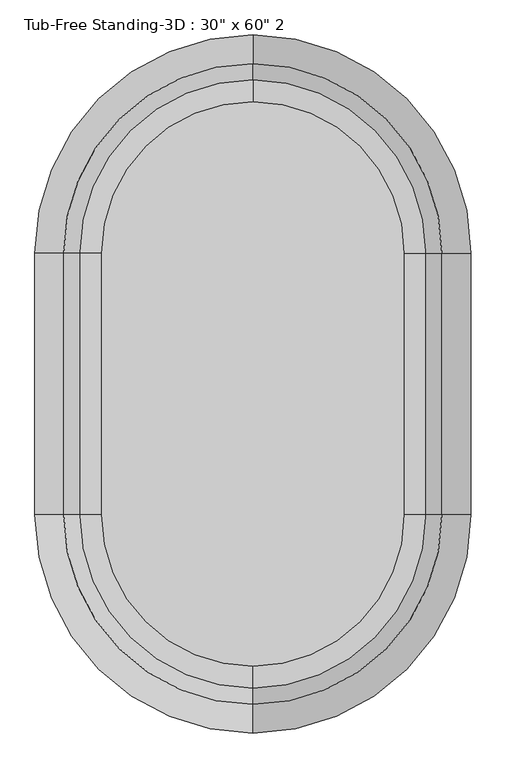
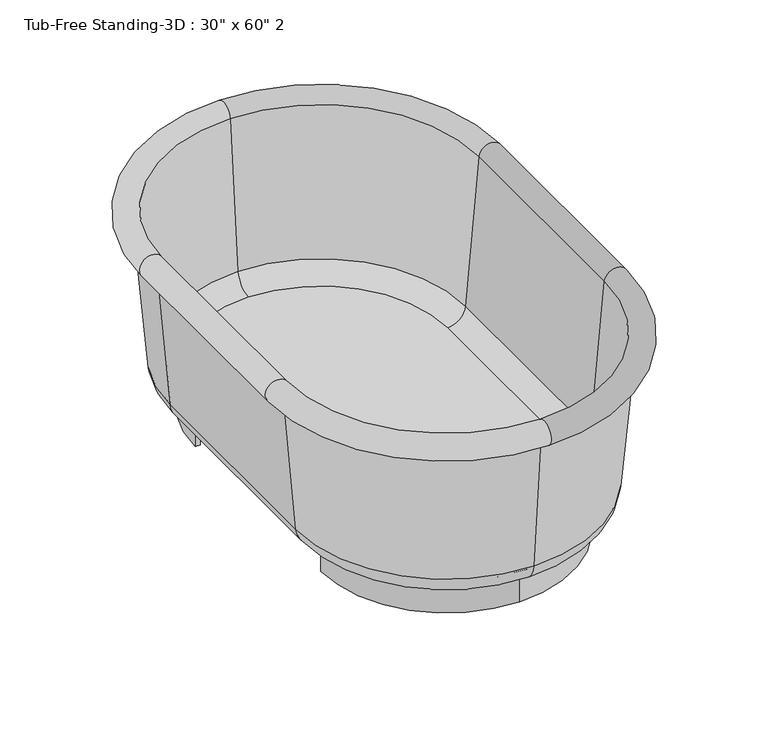
"""IFC4 building model written with IfcOpenShell, lengths in millimetres: flow terminal geometry."""

from ifc_helpers import new_model, si_unit, point, frame, frame_2d, origin, origin_with_axes, place, context, project, spatial, polyline, circle_curve, ellipse_curve, trimmed, segment, composite_curve, outline, extrude, source, transform, mapped, element, save
from ifc_brep_helpers import plane_surface, cylinder_surface, revolved_surface, advanced_brep


def flow_terminal_04541809(model_context):
    return source(origin(), model_context, "Body", "SolidModel", [
        extrude(outline(composite_curve([segment(trimmed(circle_curve(frame_2d((0.0, 228.6)), 254.0), [point((0.0, 482.6))], [point((-254.0, 228.6))], True, "CARTESIAN"), True, "CONTINUOUS"), segment(polyline([(-254.0, 228.6), (-264.2824236, 228.6)]), True, "CONTINUOUS"), segment(trimmed(circle_curve(frame_2d((0.0, 228.6)), 264.2824236), [point((-264.2824236, 228.6))], [point((0.0, 492.8824236))], False, "CARTESIAN"), True, "CONTINUOUS"), segment(trimmed(circle_curve(frame_2d((0.0, 228.6)), 264.2824236), [point((0.0, 492.8824236))], [point((264.2824236, 228.6))], False, "CARTESIAN"), True, "CONTINUOUS"), segment(polyline([(264.2824236, 228.6), (254.0, 228.6)]), True, "CONTINUOUS"), segment(trimmed(circle_curve(frame_2d((0.0, 228.6)), 254.0), [point((254.0, 228.6))], [point((0.0, 482.6))], True, "CARTESIAN"), True, "CONTINUOUS")], self_intersect=False)), origin_with_axes(), (0.0, 0.0, 1.0), 63.5),
        extrude(outline(composite_curve([segment(trimmed(circle_curve(frame_2d((0.0, -228.6)), 264.2824236), [point((0.0, -492.8824236))], [point((-264.2824236, -228.6))], False, "CARTESIAN"), True, "CONTINUOUS"), segment(polyline([(-264.2824236, -228.6), (-254.0, -228.6)]), True, "CONTINUOUS"), segment(trimmed(circle_curve(frame_2d((0.0, -228.6)), 254.0), [point((-254.0, -228.6))], [point((0.0, -482.6))], True, "CARTESIAN"), True, "CONTINUOUS"), segment(trimmed(circle_curve(frame_2d((0.0, -228.6)), 254.0), [point((0.0, -482.6))], [point((254.0, -228.6))], True, "CARTESIAN"), True, "CONTINUOUS"), segment(polyline([(254.0, -228.6), (264.2824236, -228.6)]), True, "CONTINUOUS"), segment(trimmed(circle_curve(frame_2d((0.0, -228.6)), 264.2824236), [point((264.2824236, -228.6))], [point((0.0, -492.8824236))], False, "CARTESIAN"), True, "CONTINUOUS")], self_intersect=False)), origin_with_axes(), (0.0, 0.0, 1.0), 63.5),
        extrude(outline(composite_curve([segment(polyline([(-264.2824236, -228.6), (-264.2824236, 228.6)]), True, "CONTINUOUS"), segment(trimmed(circle_curve(frame_2d((0.0, 228.6)), 264.2824236), [point((-264.2824236, 228.6))], [point((0.0, 492.8824236))], False, "CARTESIAN"), True, "CONTINUOUS"), segment(trimmed(circle_curve(frame_2d((0.0, 228.6)), 264.2824236), [point((0.0, 492.8824236))], [point((264.2824236, 228.6))], False, "CARTESIAN"), True, "CONTINUOUS"), segment(polyline([(264.2824236, 228.6), (264.2824236, -228.6)]), True, "CONTINUOUS"), segment(trimmed(circle_curve(frame_2d((0.0, -228.6)), 264.2824236), [point((264.2824236, -228.6))], [point((0.0, -492.8824236))], False, "CARTESIAN"), True, "CONTINUOUS"), segment(trimmed(circle_curve(frame_2d((0.0, -228.6)), 264.2824236), [point((0.0, -492.8824236))], [point((-264.2824236, -228.6))], False, "CARTESIAN"), True, "CONTINUOUS")], self_intersect=False)), frame((0.0, 0.0, 63.5), z_axis=(0.0, 0.0, 1.0), x_axis=(1.0, 0.0, 0.0)), (0.0, 0.0, 1.0), 15.08125),
        advanced_brep(
        [(0.0, -571.5, 406.4), (342.9, -228.6, 406.4), (355.6, -228.6, 406.4), (0.0, -584.2, 406.4), (0.0, -545.7045038, 111.5561295), (317.1045038, -228.6, 111.5561295), (0.0, -492.8824236, 63.1536107), (264.2824236, -228.6, 63.1536107), (0.0, -492.8824236, 78.0774627), (264.2824236, -228.6, 78.0774627), (0.0, -530.8374416, 112.8568289), (302.2374416, -228.6, 112.8568289), (0.0, -559.0561556, 435.3982063), (330.4561556, -228.6, 435.3982063), (-342.9, -228.6, 406.4), (-355.6, -228.6, 406.4), (-317.1045038, -228.6, 111.5561295), (-264.2824236, -228.6, 63.1536107), (-264.2824236, -228.6, 78.0774627), (-302.2374416, -228.6, 112.8568289), (-330.4561556, -228.6, 435.3982063), (-355.6, 228.6, 406.4), (-342.9, 228.6, 406.4), (-317.1045038, 228.6, 111.5561295), (-264.2824236, 228.6, 63.1536107), (-264.2824236, 228.6, 78.0774627), (-302.2374416, 228.6, 112.8568289), (-330.4561556, 228.6, 435.3982063), (0.0, 571.5, 406.4), (0.0, 584.2, 406.4), (0.0, 545.7045038, 111.5561295), (0.0, 492.8824236, 63.1536107), (0.0, 492.8824236, 78.0774627), (0.0, 530.8374416, 112.8568289), (0.0, 559.0561556, 435.3982063), (342.9, 228.6, 406.4), (355.6, 228.6, 406.4), (317.1045038, 228.6, 111.5561295), (264.2824236, 228.6, 63.1536107), (264.2824236, 228.6, 78.0774627), (302.2374416, 228.6, 112.8568289), (330.4561556, 228.6, 435.3982063)],
        [
            (0, 1, circle_curve(frame((0.0, -228.6, 406.4), z_axis=(0.0, 0.0, 1.0), x_axis=(1.0, 0.0, 0.0)), 342.9)),
            (1, 2),
            (2, 3, circle_curve(frame((0.0, -228.6, 406.4), z_axis=(0.0, 0.0, -1.0), x_axis=(1.0, 0.0, 0.0)), 355.6)),
            (3, 0),
            (4, 5, circle_curve(frame((0.0, -228.6, 111.5561295), z_axis=(0.0, 0.0, 1.0), x_axis=(1.0, 0.0, 0.0)), 317.1045038)),
            (5, 1),
            (0, 4),
            (6, 7, circle_curve(frame((0.0, -228.6, 63.1536107), z_axis=(0.0, 0.0, 1.0), x_axis=(1.0, 0.0, 0.0)), 264.2824236)),
            (7, 5, circle_curve(frame((264.2824236, -228.6, 116.1774627), z_axis=(0.0, -1.0, 0.0), x_axis=(1.0, 0.0, 0.0)), 53.023852)),
            (4, 6, circle_curve(frame((0.0, -492.8824236, 116.1774627), z_axis=(1.0, 0.0, 0.0), x_axis=(0.0, -1.0, 0.0)), 53.023852)),
            (8, 9, circle_curve(frame((0.0, -228.6, 78.0774627), z_axis=(0.0, 0.0, 1.0), x_axis=(1.0, 0.0, 0.0)), 264.2824236)),
            (9, 7),
            (6, 8),
            (10, 11, circle_curve(frame((0.0, -228.6, 112.8568289), z_axis=(0.0, 0.0, 1.0), x_axis=(1.0, 0.0, 0.0)), 302.2374416)),
            (11, 9, circle_curve(frame((264.2824236, -228.6, 116.1774627), z_axis=(0.0, 1.0, 0.0), x_axis=(1.0, 0.0, 0.0)), 38.1)),
            (8, 10, circle_curve(frame((0.0, -492.8824236, 116.1774627), z_axis=(-1.0, 0.0, 0.0), x_axis=(0.0, -1.0, 0.0)), 38.1)),
            (12, 13, circle_curve(frame((0.0, -228.6, 435.3982063), z_axis=(0.0, 0.0, 1.0), x_axis=(1.0, 0.0, 0.0)), 330.4561556)),
            (13, 11),
            (10, 12),
            (2, 13, circle_curve(frame((355.6, -228.6, 431.8), z_axis=(0.0, -1.0, 0.0), x_axis=(1.0, 0.0, 0.0)), 25.4)),
            (12, 3, circle_curve(frame((0.0, -584.2, 431.8), z_axis=(1.0, 0.0, 0.0), x_axis=(0.0, -1.0, 0.0)), 25.4)),
            (14, 0, circle_curve(frame((0.0, -228.6, 406.4), z_axis=(0.0, 0.0, 1.0), x_axis=(0.0, -1.0, 0.0)), 342.9)),
            (3, 15, circle_curve(frame((0.0, -228.6, 406.4), z_axis=(0.0, 0.0, -1.0), x_axis=(0.0, -1.0, 0.0)), 355.6)),
            (15, 14),
            (16, 4, circle_curve(frame((0.0, -228.6, 111.5561295), z_axis=(0.0, 0.0, 1.0), x_axis=(0.0, -1.0, 0.0)), 317.1045038)),
            (14, 16),
            (17, 6, circle_curve(frame((0.0, -228.6, 63.1536107), z_axis=(0.0, 0.0, 1.0), x_axis=(0.0, -1.0, 0.0)), 264.2824236)),
            (16, 17, circle_curve(frame((-264.2824236, -228.6, 116.1774627), z_axis=(0.0, -1.0, 0.0), x_axis=(-1.0, 0.0, 0.0)), 53.023852)),
            (18, 8, circle_curve(frame((0.0, -228.6, 78.0774627), z_axis=(0.0, 0.0, 1.0), x_axis=(0.0, -1.0, 0.0)), 264.2824236)),
            (17, 18),
            (19, 10, circle_curve(frame((0.0, -228.6, 112.8568289), z_axis=(0.0, 0.0, 1.0), x_axis=(0.0, -1.0, 0.0)), 302.2374416)),
            (18, 19, circle_curve(frame((-264.2824236, -228.6, 116.1774627), z_axis=(0.0, 1.0, 0.0), x_axis=(-1.0, 0.0, 0.0)), 38.1)),
            (20, 12, circle_curve(frame((0.0, -228.6, 435.3982063), z_axis=(0.0, 0.0, 1.0), x_axis=(0.0, -1.0, 0.0)), 330.4561556)),
            (19, 20),
            (20, 15, circle_curve(frame((-355.6, -228.6, 431.8), z_axis=(0.0, -1.0, 0.0), x_axis=(-1.0, 0.0, 0.0)), 25.4)),
            (15, 21),
            (21, 22),
            (22, 14),
            (22, 23),
            (23, 16),
            (23, 24, circle_curve(frame((-264.2824236, 228.6, 116.1774627), z_axis=(0.0, -1.0, 0.0), x_axis=(-1.0, 0.0, 0.0)), 53.023852)),
            (24, 17),
            (24, 25),
            (25, 18),
            (25, 26, circle_curve(frame((-264.2824236, 228.6, 116.1774627), z_axis=(0.0, 1.0, 0.0), x_axis=(-1.0, 0.0, 0.0)), 38.1)),
            (26, 19),
            (26, 27),
            (27, 20),
            (27, 21, circle_curve(frame((-355.6, 228.6, 431.8), z_axis=(0.0, -1.0, 0.0), x_axis=(-1.0, 0.0, 0.0)), 25.4)),
            (28, 22, circle_curve(frame((0.0, 228.6, 406.4), z_axis=(0.0, 0.0, 1.0), x_axis=(-1.0, 0.0, 0.0)), 342.9)),
            (21, 29, circle_curve(frame((0.0, 228.6, 406.4), z_axis=(0.0, 0.0, -1.0), x_axis=(-1.0, 0.0, 0.0)), 355.6)),
            (29, 28),
            (30, 23, circle_curve(frame((0.0, 228.6, 111.5561295), z_axis=(0.0, 0.0, 1.0), x_axis=(-1.0, 0.0, 0.0)), 317.1045038)),
            (28, 30),
            (31, 24, circle_curve(frame((0.0, 228.6, 63.1536107), z_axis=(0.0, 0.0, 1.0), x_axis=(-1.0, 0.0, 0.0)), 264.2824236)),
            (30, 31, circle_curve(frame((0.0, 492.8824236, 116.1774627), z_axis=(-1.0, 0.0, 0.0), x_axis=(0.0, 1.0, 0.0)), 53.023852)),
            (32, 25, circle_curve(frame((0.0, 228.6, 78.0774627), z_axis=(0.0, 0.0, 1.0), x_axis=(-1.0, 0.0, 0.0)), 264.2824236)),
            (31, 32),
            (33, 26, circle_curve(frame((0.0, 228.6, 112.8568289), z_axis=(0.0, 0.0, 1.0), x_axis=(-1.0, 0.0, 0.0)), 302.2374416)),
            (32, 33, circle_curve(frame((0.0, 492.8824236, 116.1774627), z_axis=(1.0, 0.0, 0.0), x_axis=(0.0, 1.0, 0.0)), 38.1)),
            (34, 27, circle_curve(frame((0.0, 228.6, 435.3982063), z_axis=(0.0, 0.0, 1.0), x_axis=(-1.0, 0.0, 0.0)), 330.4561556)),
            (33, 34),
            (34, 29, circle_curve(frame((0.0, 584.2, 431.8), z_axis=(-1.0, 0.0, 0.0), x_axis=(0.0, 1.0, 0.0)), 25.4)),
            (35, 28, circle_curve(frame((0.0, 228.6, 406.4), z_axis=(0.0, 0.0, 1.0), x_axis=(0.0, 1.0, 0.0)), 342.9)),
            (29, 36, circle_curve(frame((0.0, 228.6, 406.4), z_axis=(0.0, 0.0, -1.0), x_axis=(0.0, 1.0, 0.0)), 355.6)),
            (36, 35),
            (37, 30, circle_curve(frame((0.0, 228.6, 111.5561295), z_axis=(0.0, 0.0, 1.0), x_axis=(0.0, 1.0, 0.0)), 317.1045038)),
            (35, 37),
            (38, 31, circle_curve(frame((0.0, 228.6, 63.1536107), z_axis=(0.0, 0.0, 1.0), x_axis=(0.0, 1.0, 0.0)), 264.2824236)),
            (37, 38, circle_curve(frame((264.2824236, 228.6, 116.1774627), z_axis=(0.0, 1.0, 0.0), x_axis=(1.0, 0.0, 0.0)), 53.023852)),
            (39, 32, circle_curve(frame((0.0, 228.6, 78.0774627), z_axis=(0.0, 0.0, 1.0), x_axis=(0.0, 1.0, 0.0)), 264.2824236)),
            (38, 39),
            (40, 33, circle_curve(frame((0.0, 228.6, 112.8568289), z_axis=(0.0, 0.0, 1.0), x_axis=(0.0, 1.0, 0.0)), 302.2374416)),
            (39, 40, circle_curve(frame((264.2824236, 228.6, 116.1774627), z_axis=(0.0, -1.0, 0.0), x_axis=(1.0, 0.0, 0.0)), 38.1)),
            (41, 34, circle_curve(frame((0.0, 228.6, 435.3982063), z_axis=(0.0, 0.0, 1.0), x_axis=(0.0, 1.0, 0.0)), 330.4561556)),
            (40, 41),
            (41, 36, circle_curve(frame((355.6, 228.6, 431.8), z_axis=(0.0, 1.0, 0.0), x_axis=(1.0, 0.0, 0.0)), 25.4)),
            (36, 2),
            (1, 35),
            (5, 37),
            (7, 38),
            (9, 39),
            (11, 40),
            (13, 41),
        ],
        [
            plane_surface(frame((0.0, -228.6, 406.4), z_axis=(0.0, 0.0, -1.0), x_axis=(1.0, 0.0, 0.0))),
            revolved_surface(polyline([(342.9, -228.6, 406.4), (317.1045038, -228.6, 111.5561295)]), (0.0, -228.6, 431.8), (0.0, 0.0, -1.0)),
            revolved_surface(trimmed(ellipse_curve(frame((264.2824236, -228.6, 116.1774627), z_axis=(0.0, 1.0, 0.0), x_axis=(1.0, 0.0, 0.0)), 53.023852, 53.023852), [point((317.1045038, -228.6, 111.5561295))], [point((264.2824236, -228.6, 63.1536107))], True, "CARTESIAN"), (0.0, -228.6, 431.8), (0.0, 0.0, -1.0)),
            revolved_surface(polyline([(264.2824236, -228.6, 63.1536107), (264.2824236, -228.6, 78.07746270000001)]), (0.0, -228.6, 431.8), (0.0, 0.0, -1.0)),
            revolved_surface(trimmed(ellipse_curve(frame((264.2824236, -228.6, 116.1774627), z_axis=(0.0, -1.0, 0.0), x_axis=(1.0, 0.0, 0.0)), 38.1, 38.1), [point((264.2824236, -228.6, 78.0774627))], [point((302.2374416, -228.6, 112.8568289))], True, "CARTESIAN"), (0.0, -228.6, 431.8), (0.0, 0.0, -1.0)),
            revolved_surface(polyline([(302.2374416, -228.6, 112.8568289), (330.4561556, -228.6, 435.3982063)]), (0.0, -228.6, 431.8), (0.0, 0.0, -1.0)),
            revolved_surface(trimmed(ellipse_curve(frame((355.6, -228.6, 431.8), z_axis=(0.0, 1.0, 0.0), x_axis=(1.0, 0.0, 0.0)), 25.4, 25.4), [point((330.4561556, -228.6, 435.3982063))], [point((355.6, -228.6, 406.4))], True, "CARTESIAN"), (0.0, -228.6, 431.8), (0.0, 0.0, -1.0)),
            plane_surface(frame((0.0, -228.6, 406.4), z_axis=(0.0, 0.0, -1.0), x_axis=(0.0, -1.0, 0.0))),
            revolved_surface(polyline([(0.0, -571.5, 406.4), (0.0, -545.7045038, 111.5561295)]), (0.0, -228.6, 431.8), (0.0, 0.0, -1.0)),
            revolved_surface(trimmed(ellipse_curve(frame((0.0, -492.8824236, 116.1774627), z_axis=(1.0, 0.0, 0.0), x_axis=(0.0, -1.0, 0.0)), 53.023852, 53.023852), [point((0.0, -545.7045038, 111.5561295))], [point((0.0, -492.8824236, 63.1536107))], True, "CARTESIAN"), (0.0, -228.6, 431.8), (0.0, 0.0, -1.0)),
            revolved_surface(polyline([(0.0, -492.88242360000004, 63.1536107), (0.0, -492.88242360000004, 78.07746270000001)]), (0.0, -228.6, 431.8), (0.0, 0.0, -1.0)),
            revolved_surface(trimmed(ellipse_curve(frame((0.0, -492.8824236, 116.1774627), z_axis=(-1.0, 0.0, 0.0), x_axis=(0.0, -1.0, 0.0)), 38.1, 38.1), [point((0.0, -492.8824236, 78.0774627))], [point((0.0, -530.8374416, 112.8568289))], True, "CARTESIAN"), (0.0, -228.6, 431.8), (0.0, 0.0, -1.0)),
            revolved_surface(polyline([(0.0, -530.8374416, 112.8568289), (0.0, -559.0561556, 435.3982063)]), (0.0, -228.6, 431.8), (0.0, 0.0, -1.0)),
            revolved_surface(trimmed(ellipse_curve(frame((0.0, -584.2, 431.8), z_axis=(1.0, 0.0, 0.0), x_axis=(0.0, -1.0, 0.0)), 25.4, 25.4), [point((0.0, -559.0561556, 435.3982063))], [point((0.0, -584.2, 406.4))], True, "CARTESIAN"), (0.0, -228.6, 431.8), (0.0, 0.0, -1.0)),
            plane_surface(frame((-355.6, -228.6, 406.4), z_axis=(0.0, 0.0, -1.0), x_axis=(0.0, 1.0, 0.0))),
            plane_surface(frame((-342.9, -228.6, 406.4), z_axis=(-0.9961946980917455, 0.0, -0.08715574274765871), x_axis=(0.0, 1.0, 0.0))),
            cylinder_surface(frame((-264.2824236, -228.6, 116.1774627), z_axis=(0.0, -1.0, 0.0), x_axis=(-1.0, 0.0, 0.0)), 53.023852),
            plane_surface(frame((-264.2824236, -228.6, 63.1536107), z_axis=(1.0, 0.0, 0.0), x_axis=(0.0, 1.0, 0.0))),
            revolved_surface(polyline([(-302.38242360000004, 228.6, 116.1774627), (-302.38242360000004, -228.6, 116.1774627)]), (-264.2824236, -228.6, 116.1774627), (0.0, 1.0, 0.0)),
            plane_surface(frame((-302.2374416, -228.6, 112.8568289), z_axis=(0.9961946980917458, 0.0, 0.08715574274765651), x_axis=(0.0, 1.0, 0.0))),
            cylinder_surface(frame((-355.6, -228.6, 431.8), z_axis=(0.0, -1.0, 0.0), x_axis=(-1.0, 0.0, 0.0)), 25.4),
            plane_surface(frame((0.0, 228.6, 406.4), z_axis=(0.0, 0.0, -1.0), x_axis=(-1.0, 0.0, 0.0))),
            revolved_surface(polyline([(-342.9, 228.6, 406.4), (-317.1045038, 228.6, 111.5561295)]), (0.0, 228.6, 431.8), (0.0, 0.0, -1.0)),
            revolved_surface(trimmed(ellipse_curve(frame((-264.2824236, 228.6, 116.1774627), z_axis=(0.0, -1.0, 0.0), x_axis=(-1.0, 0.0, 0.0)), 53.023852, 53.023852), [point((-317.1045038, 228.6, 111.5561295))], [point((-264.2824236, 228.6, 63.1536107))], True, "CARTESIAN"), (0.0, 228.6, 431.8), (0.0, 0.0, -1.0)),
            revolved_surface(polyline([(-264.2824236, 228.6, 63.1536107), (-264.2824236, 228.6, 78.07746270000001)]), (0.0, 228.6, 431.8), (0.0, 0.0, -1.0)),
            revolved_surface(trimmed(ellipse_curve(frame((-264.2824236, 228.6, 116.1774627), z_axis=(0.0, 1.0, 0.0), x_axis=(-1.0, 0.0, 0.0)), 38.1, 38.1), [point((-264.2824236, 228.6, 78.0774627))], [point((-302.2374416, 228.6, 112.8568289))], True, "CARTESIAN"), (0.0, 228.6, 431.8), (0.0, 0.0, -1.0)),
            revolved_surface(polyline([(-302.2374416, 228.6, 112.8568289), (-330.4561556, 228.6, 435.3982063)]), (0.0, 228.6, 431.8), (0.0, 0.0, -1.0)),
            revolved_surface(trimmed(ellipse_curve(frame((-355.6, 228.6, 431.8), z_axis=(0.0, -1.0, 0.0), x_axis=(-1.0, 0.0, 0.0)), 25.4, 25.4), [point((-330.4561556, 228.6, 435.3982063))], [point((-355.6, 228.6, 406.4))], True, "CARTESIAN"), (0.0, 228.6, 431.8), (0.0, 0.0, -1.0)),
            plane_surface(frame((0.0, 228.6, 406.4), z_axis=(0.0, 0.0, -1.0), x_axis=(0.0, 1.0, 0.0))),
            revolved_surface(polyline([(0.0, 571.5, 406.4), (0.0, 545.7045038, 111.5561295)]), (0.0, 228.6, 431.8), (0.0, 0.0, -1.0)),
            revolved_surface(trimmed(ellipse_curve(frame((0.0, 492.8824236, 116.1774627), z_axis=(-1.0, 0.0, 0.0), x_axis=(0.0, 1.0, 0.0)), 53.023852, 53.023852), [point((0.0, 545.7045038, 111.5561295))], [point((0.0, 492.8824236, 63.1536107))], True, "CARTESIAN"), (0.0, 228.6, 431.8), (0.0, 0.0, -1.0)),
            revolved_surface(polyline([(0.0, 492.88242360000004, 63.1536107), (0.0, 492.88242360000004, 78.07746270000001)]), (0.0, 228.6, 431.8), (0.0, 0.0, -1.0)),
            revolved_surface(trimmed(ellipse_curve(frame((0.0, 492.8824236, 116.1774627), z_axis=(1.0, 0.0, 0.0), x_axis=(0.0, 1.0, 0.0)), 38.1, 38.1), [point((0.0, 492.8824236, 78.0774627))], [point((0.0, 530.8374416, 112.8568289))], True, "CARTESIAN"), (0.0, 228.6, 431.8), (0.0, 0.0, -1.0)),
            revolved_surface(polyline([(0.0, 530.8374416, 112.8568289), (0.0, 559.0561556, 435.3982063)]), (0.0, 228.6, 431.8), (0.0, 0.0, -1.0)),
            revolved_surface(trimmed(ellipse_curve(frame((0.0, 584.2, 431.8), z_axis=(-1.0, 0.0, 0.0), x_axis=(0.0, 1.0, 0.0)), 25.4, 25.4), [point((0.0, 559.0561556, 435.3982063))], [point((0.0, 584.2, 406.4))], True, "CARTESIAN"), (0.0, 228.6, 431.8), (0.0, 0.0, -1.0)),
            plane_surface(frame((355.6, 228.6, 406.4), z_axis=(0.0, 0.0, -1.0), x_axis=(0.0, -1.0, 0.0))),
            plane_surface(frame((342.9, 228.6, 406.4), z_axis=(0.9961946980917455, 0.0, -0.08715574274765871), x_axis=(0.0, -1.0, 0.0))),
            cylinder_surface(frame((264.2824236, 228.6, 116.1774627), z_axis=(0.0, 1.0, 0.0), x_axis=(1.0, 0.0, 0.0)), 53.023852),
            plane_surface(frame((264.2824236, 228.6, 63.1536107), z_axis=(-1.0, 0.0, 0.0), x_axis=(0.0, -1.0, 0.0))),
            revolved_surface(polyline([(302.38242360000004, -228.6, 116.1774627), (302.38242360000004, 228.6, 116.1774627)]), (264.2824236, 228.6, 116.1774627), (0.0, -1.0, 0.0)),
            plane_surface(frame((302.2374416, 228.6, 112.8568289), z_axis=(-0.9961946980917458, 0.0, 0.08715574274765651), x_axis=(0.0, -1.0, 0.0))),
            cylinder_surface(frame((355.6, 228.6, 431.8), z_axis=(0.0, 1.0, 0.0), x_axis=(1.0, 0.0, 0.0)), 25.4),
        ],
        [
            (0, [[1, 2, 3, 4]]),
            (1, [[5, 6, -1, 7]]),
            (2, [[8, 9, -5, 10]]),
            (3, [[11, 12, -8, 13]]),
            (4, [[14, 15, -11, 16]]),
            (5, [[17, 18, -14, 19]]),
            (6, [[-3, 20, -17, 21]]),
            (7, [[22, -4, 23, 24]]),
            (8, [[25, -7, -22, 26]]),
            (9, [[27, -10, -25, 28]]),
            (10, [[29, -13, -27, 30]]),
            (11, [[31, -16, -29, 32]]),
            (12, [[33, -19, -31, 34]]),
            (13, [[-23, -21, -33, 35]]),
            (14, [[-24, 36, 37, 38]]),
            (15, [[-26, -38, 39, 40]]),
            (16, [[-28, -40, 41, 42]]),
            (17, [[-30, -42, 43, 44]]),
            (18, [[-32, -44, 45, 46]]),
            (19, [[-34, -46, 47, 48]]),
            (20, [[-35, -48, 49, -36]]),
            (21, [[50, -37, 51, 52]]),
            (22, [[53, -39, -50, 54]]),
            (23, [[55, -41, -53, 56]]),
            (24, [[57, -43, -55, 58]]),
            (25, [[59, -45, -57, 60]]),
            (26, [[61, -47, -59, 62]]),
            (27, [[-51, -49, -61, 63]]),
            (28, [[64, -52, 65, 66]]),
            (29, [[67, -54, -64, 68]]),
            (30, [[69, -56, -67, 70]]),
            (31, [[71, -58, -69, 72]]),
            (32, [[73, -60, -71, 74]]),
            (33, [[75, -62, -73, 76]]),
            (34, [[-65, -63, -75, 77]]),
            (35, [[-66, 78, -2, 79]]),
            (36, [[-68, -79, -6, 80]]),
            (37, [[-70, -80, -9, 81]]),
            (38, [[-72, -81, -12, 82]]),
            (39, [[-74, -82, -15, 83]]),
            (40, [[-76, -83, -18, 84]]),
            (41, [[-77, -84, -20, -78]]),
        ],
    ),
    ])


if __name__ == "__main__":
    model = new_model("IFC4")
    model_context = context("Model", 3, world=origin())
    ifc_project = project(units=[si_unit("LENGTHUNIT", "METRE", prefix="MILLI")], contexts=[model_context])
    site = spatial("IfcSite", under=ifc_project)
    building = spatial("IfcBuilding", under=site)
    placement = place(None, origin())
    flow_terminal_shape = flow_terminal_04541809(model_context)
    element("IfcFlowTerminal", 1, ObjectType="Tub-Free Standing-3D : 30\" x 60\" 2", at=placement, inside=building, context=model_context, shape_type="MappedRepresentation", body=[
        mapped(flow_terminal_shape, transform((0.0, 0.0, 0.0), x_axis=(1.0, 0.0, 0.0), y_axis=(0.0, 1.0, 0.0), z_axis=(0.0, 0.0, 1.0))),
    ])
    save(model, "model.ifc")

# Revit data of these elements
# Type "Tub-Free Standing-3D : 30\" x 60\" 2"
#   Assembly Code = "D2010110"
#   Height = 1' - 6"
#   Length = 4' - 0"
#   Width = 2' - 6"
#   Tub Material = Porcelain, Ivory
#   Default Elevation = 0
# Element 1 (IfcFlowTerminal, "Tub-Free Standing-3D : 30\" x 60\" 2")
#   Materials on its faces: "Porcelain, Ivory"
# Materials
#   "Porcelain, Ivory": class "Ceramic", colour RGB 247 247 239, transparency 0, Description = "Porcelain, ivory", Cost = 0
